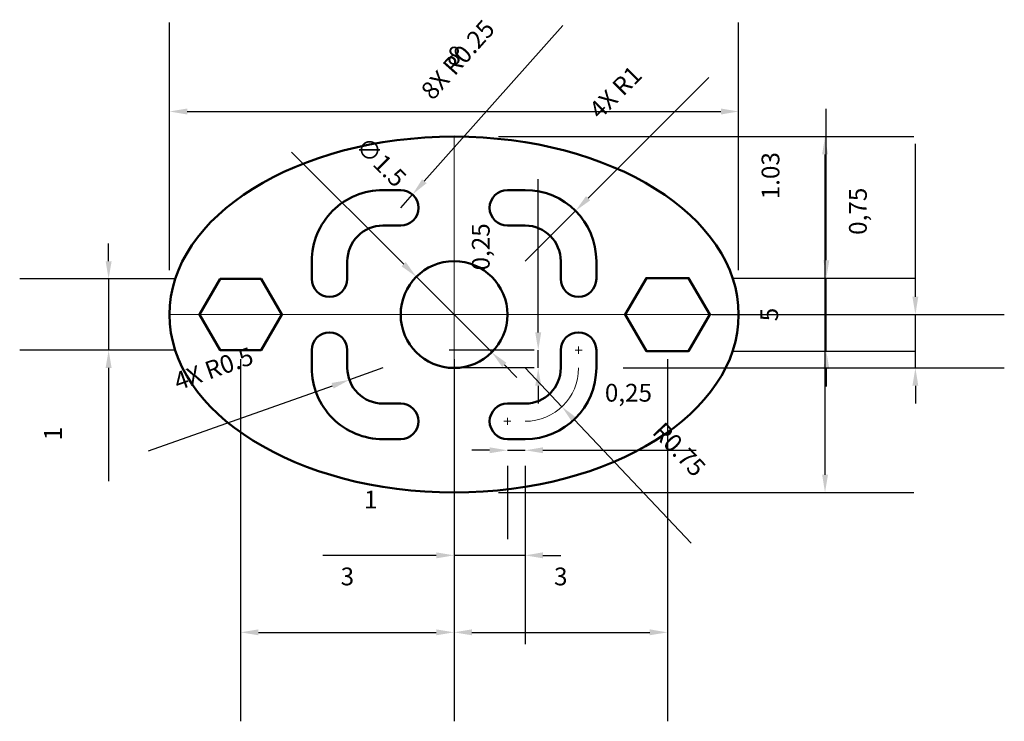
# Model space of a CAD drawing. Units: millimetres. Extents: x 1504.9 to 1518.7, y 1474.3 to 1484.2.
import ezdxf

# ---------------------------------------------------------------- set-up
doc = ezdxf.new("R2010")
doc.units = ezdxf.units.MM
doc.linetypes.add('CENTER', pattern=[50.8, 31.75, -6.35, 6.35, -6.35])
for name, color, linetype, lineweight in [('M-CNTR', 4, 'CENTER', 18), ('M-CONS', 8, 'Continuous', 13), ('M-DIMS', 2, 'Continuous', 25), ('M-OUTL', 7, 'Continuous', 50)]:
    doc.layers.add(name, color=color, linetype=linetype, lineweight=lineweight)
doc.styles.get("Standard").update_dxf_attribs({"font": 'arial.ttf'})
doc.dimstyles.new('ISO-25', dxfattribs={"dimtxt": 0.25, "dimasz": 0.25, "dimexe": 1.25, "dimexo": 0.625, "dimtad": 1, "dimtxsty": 'Standard', "dimcen": 2.5, "dimadec": 0, "dimazin": 0, "dimtfac": 1, "dimtmove": 0, "dimatfit": 3, "dimfxl": 1, "dimarcsym": 0})

# ---------------------------------------------------------------- blocks, each defined once
blk = doc.blocks.new('*D1')
at = {"layer": 'Defpoints', "color": 0, "transparency": 16777216}
for p in [(1507.987, 1480.057), (1510.987, 1480.057), (1510.987, 1475.592)]:
    blk.add_point(p, dxfattribs=at)
at = {"layer": 'M-DIMS', "color": 0, "lineweight": -2, "transparency": 16777216}
for p, q in [((1507.987, 1479.432), (1507.987, 1474.342)), ((1510.987, 1479.432), (1510.987, 1474.342)), ((1508.237, 1475.592), (1510.737, 1475.592))]:
    blk.add_line(p, q, dxfattribs=at)
at = {"layer": 'M-DIMS', "color": 0, "transparency": 16777216}
for points in [[(1508.237, 1475.634), (1508.237, 1475.551), (1507.987, 1475.592)], [(1510.737, 1475.634), (1510.737, 1475.551), (1510.987, 1475.592)]]:
    blk.add_solid(points, dxfattribs=at)
at = {"layer": 'M-DIMS', "color": 0, "transparency": 16777216, "insert": (1509.487, 1476.345), "char_height": 0.25, "attachment_point": 5}
blk.add_mtext('3', dxfattribs=at)
blk = doc.blocks.new('*D2')
at = {"layer": 'Defpoints', "color": 0, "transparency": 16777216}
for p in [(1510.987, 1480.057), (1513.987, 1480.057), (1513.987, 1475.592)]:
    blk.add_point(p, dxfattribs=at)
at = {"layer": 'M-DIMS', "color": 0, "lineweight": -2, "transparency": 16777216}
for p, q in [((1510.987, 1479.432), (1510.987, 1474.342)), ((1513.987, 1479.432), (1513.987, 1474.342)), ((1511.237, 1475.592), (1513.737, 1475.592))]:
    blk.add_line(p, q, dxfattribs=at)
at = {"layer": 'M-DIMS', "color": 0, "transparency": 16777216}
for points in [[(1511.237, 1475.634), (1511.237, 1475.551), (1510.987, 1475.592)], [(1513.737, 1475.634), (1513.737, 1475.551), (1513.987, 1475.592)]]:
    blk.add_solid(points, dxfattribs=at)
at = {"layer": 'M-DIMS', "color": 0, "transparency": 16777216, "insert": (1512.487, 1476.345), "char_height": 0.25, "attachment_point": 5}
blk.add_mtext('3', dxfattribs=at)
blk = doc.blocks.new('*D3')
at = {"layer": 'Defpoints', "color": 0, "transparency": 16777216}
for p in [(1510.987, 1482.557), (1516.201, 1482.557), (1510.987, 1477.557)]:
    blk.add_point(p, dxfattribs=at)
at = {"layer": 'M-DIMS', "color": 0, "lineweight": -2, "transparency": 16777216}
for p, q in [((1511.612, 1482.557), (1517.451, 1482.557)), ((1516.201, 1477.807), (1516.201, 1482.307)), ((1511.612, 1477.557), (1517.451, 1477.557))]:
    blk.add_line(p, q, dxfattribs=at)
at = {"layer": 'M-DIMS', "color": 0, "transparency": 16777216}
for points in [[(1516.16, 1482.307), (1516.243, 1482.307), (1516.201, 1482.557)], [(1516.16, 1477.807), (1516.243, 1477.807), (1516.201, 1477.557)]]:
    blk.add_solid(points, dxfattribs=at)
at = {"layer": 'M-DIMS', "color": 0, "transparency": 16777216, "insert": (1515.449, 1480.057), "char_height": 0.25, "attachment_point": 5, "rotation": 90}
blk.add_mtext('5', dxfattribs=at)
blk = doc.blocks.new('*D4')
at = {"layer": 'Defpoints', "color": 0, "transparency": 16777216}
for p in [(1514.987, 1482.91), (1506.987, 1480.057), (1514.987, 1480.057)]:
    blk.add_point(p, dxfattribs=at)
at = {"layer": 'M-DIMS', "color": 0, "lineweight": -2, "transparency": 16777216}
for p, q in [((1506.987, 1480.682), (1506.987, 1484.16)), ((1514.987, 1480.682), (1514.987, 1484.16)), ((1507.237, 1482.91), (1514.737, 1482.91))]:
    blk.add_line(p, q, dxfattribs=at)
at = {"layer": 'M-DIMS', "color": 0, "transparency": 16777216}
for points in [[(1507.237, 1482.952), (1507.237, 1482.868), (1506.987, 1482.91)], [(1514.737, 1482.952), (1514.737, 1482.868), (1514.987, 1482.91)]]:
    blk.add_solid(points, dxfattribs=at)
at = {"layer": 'M-DIMS', "color": 0, "transparency": 16777216, "insert": (1510.987, 1483.663), "char_height": 0.25, "attachment_point": 5}
blk.add_mtext('8', dxfattribs=at)
blk = doc.blocks.new('*D5')
at = {"layer": 'Defpoints', "color": 0, "transparency": 16777216}
for p in [(1507.698, 1480.557), (1506.132, 1479.557), (1507.698, 1479.557)]:
    blk.add_point(p, dxfattribs=at)
at = {"layer": 'M-DIMS', "color": 0, "lineweight": -2, "transparency": 16777216}
for p, q in [((1506.132, 1480.807), (1506.132, 1481.057)), ((1507.073, 1480.557), (1504.882, 1480.557)), ((1506.132, 1480.557), (1506.132, 1479.557)), ((1507.073, 1479.557), (1504.882, 1479.557)), ((1506.132, 1479.307), (1506.132, 1477.714))]:
    blk.add_line(p, q, dxfattribs=at)
at = {"layer": 'M-DIMS', "color": 0, "transparency": 16777216}
for points in [[(1506.09, 1480.807), (1506.174, 1480.807), (1506.132, 1480.557)], [(1506.09, 1479.307), (1506.174, 1479.307), (1506.132, 1479.557)]]:
    blk.add_solid(points, dxfattribs=at)
at = {"layer": 'M-DIMS', "color": 0, "transparency": 16777216, "insert": (1505.382, 1478.385), "char_height": 0.25, "attachment_point": 5, "rotation": 90}
blk.add_mtext('1', dxfattribs=at)
blk = doc.blocks.new('*D6')
at = {"layer": 'Defpoints', "color": 0, "transparency": 16777216}
for p in [(1511.737, 1478.557), (1511.987, 1478.557), (1511.987, 1478.15)]:
    blk.add_point(p, dxfattribs=at)
at = {"layer": 'M-DIMS', "color": 0, "lineweight": -2, "transparency": 16777216}
for p, q in [((1511.487, 1478.15), (1511.237, 1478.15)), ((1511.737, 1478.15), (1511.987, 1478.15)), ((1512.237, 1478.15), (1514.388, 1478.15)), ((1511.737, 1477.932), (1511.737, 1476.9)), ((1511.987, 1477.932), (1511.987, 1476.9))]:
    blk.add_line(p, q, dxfattribs=at)
at = {"layer": 'M-DIMS', "color": 0, "transparency": 16777216}
for points in [[(1511.487, 1478.192), (1511.487, 1478.109), (1511.737, 1478.15)], [(1512.237, 1478.192), (1512.237, 1478.109), (1511.987, 1478.15)]]:
    blk.add_solid(points, dxfattribs=at)
at = {"layer": 'M-DIMS', "color": 0, "transparency": 16777216, "insert": (1513.438, 1478.926), "char_height": 0.25, "attachment_point": 5}
blk.add_mtext('0,25', dxfattribs=at)
blk = doc.blocks.new('*D7')
at = {"layer": 'Defpoints', "color": 0, "transparency": 16777216}
for p in [(1512.17, 1479.557), (1512.737, 1479.557), (1512.737, 1479.307)]:
    blk.add_point(p, dxfattribs=at)
at = {"layer": 'M-DIMS', "color": 0, "lineweight": -2, "transparency": 16777216}
for p, q in [((1512.17, 1479.807), (1512.17, 1481.958)), ((1512.112, 1479.557), (1510.92, 1479.557)), ((1512.17, 1479.307), (1512.17, 1479.557)), ((1512.112, 1479.307), (1510.92, 1479.307)), ((1512.17, 1479.057), (1512.17, 1478.807))]:
    blk.add_line(p, q, dxfattribs=at)
at = {"layer": 'M-DIMS', "color": 0, "transparency": 16777216}
for points in [[(1512.128, 1479.807), (1512.212, 1479.807), (1512.17, 1479.557)], [(1512.128, 1479.057), (1512.212, 1479.057), (1512.17, 1479.307)]]:
    blk.add_solid(points, dxfattribs=at)
at = {"layer": 'M-DIMS', "color": 0, "transparency": 16777216, "insert": (1511.395, 1481.008), "char_height": 0.25, "attachment_point": 5, "rotation": 90}
blk.add_mtext('0,25', dxfattribs=at)
blk = doc.blocks.new('*D8')
at = {"layer": 'Defpoints', "color": 0, "transparency": 16777216}
for p in [(1510.987, 1478.557), (1511.987, 1478.557), (1510.987, 1476.674)]:
    blk.add_point(p, dxfattribs=at)
at = {"layer": 'M-DIMS', "color": 0, "lineweight": -2, "transparency": 16777216}
for p, q in [((1510.987, 1477.932), (1510.987, 1475.424)), ((1511.987, 1477.932), (1511.987, 1475.424)), ((1510.737, 1476.674), (1509.145, 1476.674)), ((1511.987, 1476.674), (1510.987, 1476.674)), ((1512.237, 1476.674), (1512.487, 1476.674))]:
    blk.add_line(p, q, dxfattribs=at)
at = {"layer": 'M-DIMS', "color": 0, "transparency": 16777216}
for points in [[(1510.737, 1476.716), (1510.737, 1476.632), (1510.987, 1476.674)], [(1512.237, 1476.716), (1512.237, 1476.632), (1511.987, 1476.674)]]:
    blk.add_solid(points, dxfattribs=at)
at = {"layer": 'M-DIMS', "color": 0, "transparency": 16777216, "insert": (1509.816, 1477.425), "char_height": 0.25, "attachment_point": 5}
blk.add_mtext('1', dxfattribs=at)
blk = doc.blocks.new('*D9')
at = {"layer": 'Defpoints', "color": 0, "transparency": 16777216}
for p in [(1513.987, 1480.057), (1517.471, 1480.057), (1512.737, 1479.307)]:
    blk.add_point(p, dxfattribs=at)
at = {"layer": 'M-DIMS', "color": 0, "lineweight": -2, "transparency": 16777216}
for p, q in [((1517.471, 1480.307), (1517.471, 1482.458)), ((1514.612, 1480.057), (1518.721, 1480.057)), ((1517.471, 1479.307), (1517.471, 1480.057)), ((1513.362, 1479.307), (1518.721, 1479.307)), ((1517.471, 1479.057), (1517.471, 1478.807))]:
    blk.add_line(p, q, dxfattribs=at)
at = {"layer": 'M-DIMS', "color": 0, "transparency": 16777216}
for points in [[(1517.429, 1480.307), (1517.512, 1480.307), (1517.471, 1480.057)], [(1517.429, 1479.057), (1517.512, 1479.057), (1517.471, 1479.307)]]:
    blk.add_solid(points, dxfattribs=at)
at = {"layer": 'M-DIMS', "color": 0, "transparency": 16777216, "insert": (1516.695, 1481.508), "char_height": 0.25, "attachment_point": 5, "rotation": 90}
blk.add_mtext('0,75', dxfattribs=at)
blk = doc.blocks.new('SLOT-QUARTER-TURN')
for p, q in [((1, 1), (1, 1.25)), ((1.5, 1), (1.5, 1.25)), ((0.5, 0.5), (0.25, 0.5)), ((0.5, 0), (0.25, 0))]:
    blk.add_line(p, q)
for centre, radius, start, end in [((1.25, 1.25), 0.25, 0, 180), ((0.5, 1), 0.5, 270, 0), ((0.5, 1), 1, 270, 0), ((0.25, 0.25), 0.25, 90, 270)]:
    blk.add_arc(centre, radius, start, end)
blk = doc.blocks.new('SLOT-END-CENTRE-MARK')
for q in [(0, 0.05), (0.05, 0.1), (0.05, 0), (0.1, 0.05)]:
    blk.add_line((0.05, 0.05), q)
blk = doc.blocks.new('*D12')
at = {"layer": 'Defpoints', "color": 0, "transparency": 16777216}
for p in [(1514.283, 1480.57), (1516.219, 1480.57), (1514.283, 1479.544)]:
    blk.add_point(p, dxfattribs=at)
at = {"layer": 'M-DIMS', "color": 0, "lineweight": -2, "transparency": 16777216}
for p, q in [((1516.219, 1480.82), (1516.219, 1482.946)), ((1514.908, 1480.57), (1517.469, 1480.57)), ((1516.219, 1479.544), (1516.219, 1480.57)), ((1514.908, 1479.544), (1517.469, 1479.544)), ((1516.219, 1479.294), (1516.219, 1479.044))]:
    blk.add_line(p, q, dxfattribs=at)
at = {"layer": 'M-DIMS', "color": 0, "transparency": 16777216}
for points in [[(1516.178, 1480.82), (1516.261, 1480.82), (1516.219, 1480.57)], [(1516.178, 1479.294), (1516.261, 1479.294), (1516.219, 1479.544)]]:
    blk.add_solid(points, dxfattribs=at)
at = {"layer": 'M-DIMS', "color": 0, "transparency": 16777216, "insert": (1515.467, 1482.008), "char_height": 0.25, "attachment_point": 5, "rotation": 90}
blk.add_mtext('1.03', dxfattribs=at)
blk = doc.blocks.new('*D13')
at = {"layer": 'Defpoints', "color": 0, "transparency": 16777216}
for p in [(1510.457, 1480.587), (1511.517, 1479.527)]:
    blk.add_point(p, dxfattribs=at)
at = {"layer": 'M-DIMS', "color": 0, "lineweight": -2, "transparency": 16777216}
for p, q in [((1508.704, 1482.34), (1510.28, 1480.764)), ((1511.517, 1479.527), (1510.457, 1480.587)), ((1511.694, 1479.35), (1511.871, 1479.173))]:
    blk.add_line(p, q, dxfattribs=at)
at = {"layer": 'M-DIMS', "color": 0, "transparency": 16777216}
for points in [[(1510.309, 1480.794), (1510.25, 1480.735), (1510.457, 1480.587)], [(1511.723, 1479.379), (1511.664, 1479.32), (1511.517, 1479.527)]]:
    blk.add_solid(points, dxfattribs=at)
at = {"layer": 'M-DIMS', "color": 0, "transparency": 16777216, "insert": (1509.941, 1482.178), "char_height": 0.25, "attachment_point": 5, "rotation": 314.9923}
blk.add_mtext('∅1.5', dxfattribs=at)
blk = doc.blocks.new('*D14')
at = {"layer": 'Defpoints', "color": 0, "transparency": 16777216}
for p in [(1512.694, 1481.514), (1511.987, 1480.807)]:
    blk.add_point(p, dxfattribs=at)
at = {"layer": 'M-DIMS', "color": 0, "lineweight": -2, "transparency": 16777216}
for p, q in [((1514.569, 1483.389), (1512.871, 1481.691)), ((1511.987, 1480.807), (1512.694, 1481.514))]:
    blk.add_line(p, q, dxfattribs=at)
at = {"layer": 'M-DIMS', "color": 0, "transparency": 16777216}
blk.add_solid([(1512.841, 1481.72), (1512.9, 1481.661), (1512.694, 1481.514)], dxfattribs=at)
at = {"layer": 'M-DIMS', "color": 0, "transparency": 16777216, "insert": (1513.278, 1483.159), "char_height": 0.25, "attachment_point": 5, "rotation": 45.0009}
blk.add_mtext('4X R1', dxfattribs=at)
blk = doc.blocks.new('*D15')
at = {"layer": 'Defpoints', "color": 0, "transparency": 16777216}
for p in [(1509.987, 1479.307), (1509.516, 1479.14)]:
    blk.add_point(p, dxfattribs=at)
at = {"layer": 'M-DIMS', "color": 0, "lineweight": -2, "transparency": 16777216}
for p, q in [((1509.987, 1479.307), (1509.516, 1479.14)), ((1506.693, 1478.142), (1509.28, 1479.057))]:
    blk.add_line(p, q, dxfattribs=at)
at = {"layer": 'M-DIMS', "color": 0, "transparency": 16777216}
blk.add_solid([(1509.266, 1479.096), (1509.294, 1479.018), (1509.516, 1479.14)], dxfattribs=at)
at = {"layer": 'M-DIMS', "color": 0, "transparency": 16777216, "insert": (1507.618, 1479.267), "char_height": 0.25, "attachment_point": 5, "rotation": 19.4779}
blk.add_mtext('4X R0.5', dxfattribs=at)
blk = doc.blocks.new('*D16')
at = {"layer": 'Defpoints', "color": 0, "transparency": 16777216}
for p in [(1510.403, 1481.744), (1510.237, 1481.557)]:
    blk.add_point(p, dxfattribs=at)
at = {"layer": 'M-DIMS', "color": 0, "lineweight": -2, "transparency": 16777216}
for p, q in [((1512.517, 1484.117), (1510.569, 1481.93)), ((1510.237, 1481.557), (1510.403, 1481.744))]:
    blk.add_line(p, q, dxfattribs=at)
at = {"layer": 'M-DIMS', "color": 0, "transparency": 16777216}
blk.add_solid([(1510.538, 1481.958), (1510.601, 1481.903), (1510.403, 1481.744)], dxfattribs=at)
at = {"layer": 'M-DIMS', "color": 0, "transparency": 16777216, "insert": (1511.064, 1483.617), "char_height": 0.25, "attachment_point": 5, "rotation": 48.3104}
blk.add_mtext('8X R0.25', dxfattribs=at)
blk = doc.blocks.new('*D17')
at = {"layer": 'Defpoints', "color": 0, "transparency": 16777216}
for p in [(1511.987, 1479.307), (1512.503, 1478.762)]:
    blk.add_point(p, dxfattribs=at)
at = {"layer": 'M-DIMS', "color": 0, "lineweight": -2, "transparency": 16777216}
for p, q in [((1511.987, 1479.307), (1512.503, 1478.762)), ((1514.318, 1476.845), (1512.674, 1478.581))]:
    blk.add_line(p, q, dxfattribs=at)
at = {"layer": 'M-DIMS', "color": 0, "transparency": 16777216}
blk.add_solid([(1512.705, 1478.609), (1512.644, 1478.552), (1512.503, 1478.762)], dxfattribs=at)
at = {"layer": 'M-DIMS', "color": 0, "transparency": 16777216, "insert": (1514.129, 1478.139), "char_height": 0.25, "attachment_point": 5, "rotation": 313.4331}
blk.add_mtext('R0.75', dxfattribs=at)

msp = doc.modelspace()

# ---------------------------------------------------------------- linework, layer by layer
at = {"layer": 'M-CNTR', "ltscale": 0.25}
for p, q in [((1510.987, 1479.307), (1510.987, 1482.557)), ((1506.987, 1480.057), (1514.987, 1480.057))]:
    msp.add_line(p, q, dxfattribs=at)
at = {"layer": 'M-CNTR', "transparency": 33554534}
msp.add_arc((1511.987, 1479.307), 0.75, 270, 0, dxfattribs=at)
at = {"layer": 'M-CONS'}
for centre, radius, start, end in [((1511.987, 1479.307), 0.75, 109.4712, 109.5728), ((1511.737, 1478.557), 0.25, 0, 1.78216911e-08)]:
    msp.add_arc(centre, radius, start, end, dxfattribs=at)
at = {"layer": 'M-OUTL'}
for points in [[(1507.698, 1480.557), (1507.409, 1480.057), (1507.698, 1479.557), (1508.276, 1479.557), (1508.565, 1480.057), (1508.275, 1480.557)], [(1514.58, 1480.057), (1514.283, 1480.57), (1513.691, 1480.57), (1513.394, 1480.057), (1513.691, 1479.544), (1514.283, 1479.544)]]:
    msp.add_lwpolyline(points, close=True, dxfattribs=at)
msp.add_circle((1510.987, 1480.057), 0.75, dxfattribs=at)
msp.add_ellipse((1510.987, 1480.057), major_axis=(-4, 0), ratio=0.625, dxfattribs=at)

# ---------------------------------------------------------------- block references
at = {"layer": 'M-CNTR'}
msp.add_blockref('SLOT-END-CENTRE-MARK', (1512.687, 1479.507), dxfattribs=at)
at = {"layer": 'M-CNTR', "rotation": 180}
msp.add_blockref('SLOT-END-CENTRE-MARK', (1511.787, 1478.607), dxfattribs=at)
at = {"layer": 'M-OUTL'}
for p, rotation in [((1510.487, 1481.807), 180), ((1512.987, 1480.307), 89.99999999996137), ((1508.987, 1479.807), 269.9999999999325)]:
    msp.add_blockref('SLOT-QUARTER-TURN', p, dxfattribs=dict(at, rotation=rotation))
msp.add_blockref('SLOT-QUARTER-TURN', (1511.487, 1478.307), dxfattribs=at)

# ---------------------------------------------------------------- dimensions: what is measured, and where the dimension line sits
at = {"layer": 'M-DIMS'}
for center, mpoint, text, override, picture, middle in [((1510.237, 1481.557), (1510.403, 1481.744), '8X <>', {"dimdec": 2, "dimlfac": 1, "dimrnd": 0, "dimzin": 0, "dimdsep": 46, "dimlunit": 2}, '*D16', (1511.064, 1483.617)), ((1511.987, 1480.807), (1512.694, 1481.514), '4X <>', {"dimdec": 0, "dimlfac": 1, "dimrnd": 0, "dimzin": 0, "dimdsep": 46, "dimlunit": 2}, '*D14', (1513.278, 1483.159)), ((1509.987, 1479.307), (1509.516, 1479.14), '4X <>', {"dimdec": 1, "dimlfac": 1, "dimrnd": 0, "dimzin": 0, "dimdsep": 46, "dimlunit": 2}, '*D15', (1507.618, 1479.267))]:
    dim = msp.add_radius_dim(center=center, mpoint=mpoint, text=text, dimstyle='ISO-25', override=override, dxfattribs=at)
    dim.commit()
    dim.dimension.update_dxf_attribs({"geometry": picture, "text_midpoint": middle})
for base, p1, p2, picture, middle in [((1514.987, 1482.91), (1506.987, 1480.057), (1514.987, 1480.057), '*D4', (1510.987, 1483.663)), ((1510.987, 1475.592), (1507.987, 1480.057), (1510.987, 1480.057), '*D1', (1509.487, 1476.345)), ((1513.987, 1475.592), (1510.987, 1480.057), (1513.987, 1480.057), '*D2', (1512.487, 1476.345)), ((1511.987, 1478.15), (1511.737, 1478.557), (1511.987, 1478.557), '*D6', (1513.438, 1478.926)), ((1510.987, 1476.674), (1511.987, 1478.557), (1510.987, 1478.557), '*D8', (1509.816, 1477.425))]:
    dim = msp.add_linear_dim(base=base, p1=p1, p2=p2, dimstyle='ISO-25', override={"dimclrd": 0, "dimclre": 0, "dimclrt": 0}, dxfattribs=at)
    dim.commit()
    dim.dimension.update_dxf_attribs({"geometry": picture, "text_midpoint": middle})
for base, p1, p2, override, picture, middle in [((1516.219, 1480.57), (1514.283, 1479.544), (1514.283, 1480.57), {"dimdec": 2, "dimlfac": 1, "dimrnd": 0, "dimzin": 0, "dimdsep": 46, "dimlunit": 2}, '*D12', (1515.467, 1482.008)), ((1516.201, 1482.557), (1510.987, 1477.557), (1510.987, 1482.557), {"dimclrd": 0, "dimclre": 0, "dimclrt": 0}, '*D3', (1515.449, 1480.057)), ((1517.471, 1480.057), (1512.737, 1479.307), (1513.987, 1480.057), {"dimclrd": 0, "dimclre": 0, "dimclrt": 0}, '*D9', (1516.695, 1481.508)), ((1512.17, 1479.557), (1512.737, 1479.307), (1512.737, 1479.557), {"dimclrd": 0, "dimclre": 0, "dimclrt": 0}, '*D7', (1511.395, 1481.008)), ((1506.132, 1479.557), (1507.698, 1480.557), (1507.698, 1479.557), {"dimclrd": 0, "dimclre": 0, "dimclrt": 0}, '*D5', (1505.382, 1478.385))]:
    dim = msp.add_linear_dim(base=base, p1=p1, p2=p2, angle=90, dimstyle='ISO-25', override=override, dxfattribs=at)
    dim.commit()
    dim.dimension.update_dxf_attribs({"geometry": picture, "text_midpoint": middle})
dim = msp.add_diameter_dim_2p(p1=(1511.517, 1479.527), p2=(1510.457, 1480.587), dimstyle='ISO-25', override={"dimdec": 1, "dimlfac": 1, "dimrnd": 0, "dimzin": 0, "dimdsep": 46, "dimlunit": 2}, dxfattribs=at)
dim.commit()
dim.dimension.update_dxf_attribs({"geometry": '*D13', "text_midpoint": (1509.404, 1481.641), "dimtype": 163})
dim = msp.add_radius_dim(center=(1511.987, 1479.307), mpoint=(1512.503, 1478.762), dimstyle='ISO-25', override={"dimdec": 2, "dimlfac": 1, "dimrnd": 0, "dimzin": 0, "dimdsep": 46, "dimlunit": 2}, dxfattribs=at)
dim.commit()
dim.dimension.update_dxf_attribs({"geometry": '*D17', "text_midpoint": (1514.129, 1478.139)})

doc.saveas('drawing.dxf')
